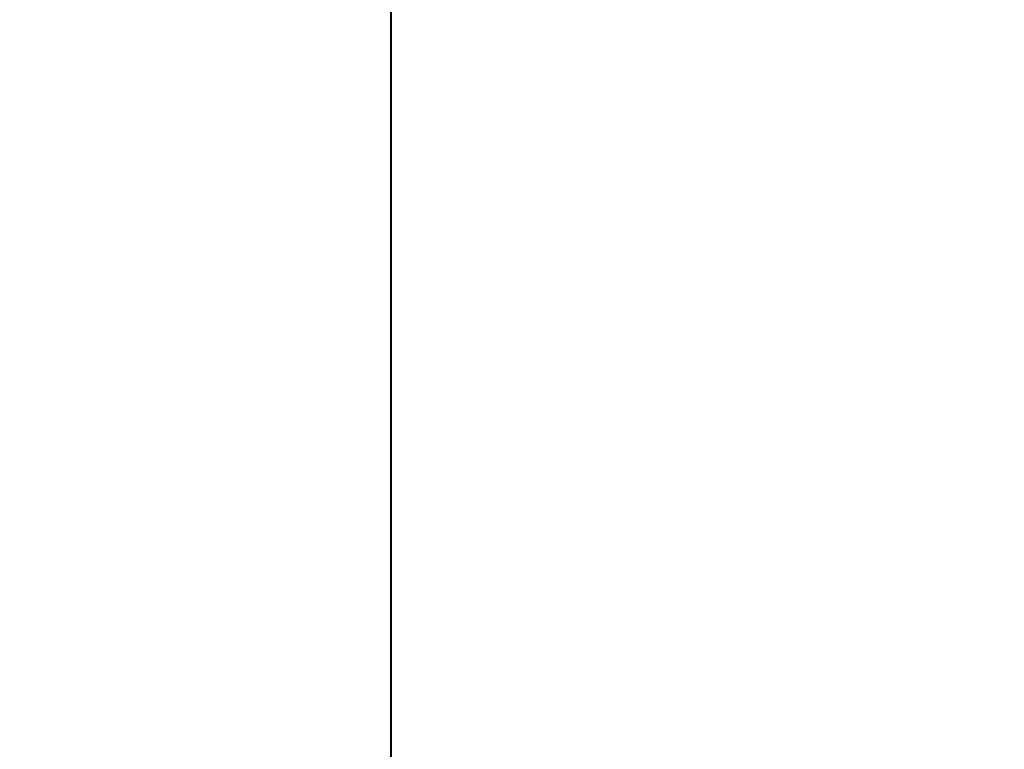
# Model space of a CAD drawing. Units: inches. Extents: x 459864 to 460310, y 324185 to 324787.
# Tile 84 of 112: x 460247.113242 to 460247.117712, y 324283.485489 to 324283.488802. Entities that reach past the tile are written whole.
import ezdxf

# ---------------------------------------------------------------- set-up
doc = ezdxf.new("R2010")
doc.units = ezdxf.units.IN
doc.layers.add('A-ANNO-DIMS', color=2, linetype='Continuous', lineweight=18)
doc.layers.add('A-WALL', color=7, linetype='Continuous', lineweight=40)
doc.styles.get("Standard").update_dxf_attribs({"font": 'arial.ttf'})
doc.dimstyles.new('ISO-25', dxfattribs={"dimtxt": 6, "dimasz": 2.5, "dimexe": 1.25, "dimexo": 0.625, "dimtad": 1, "dimdec": 1, "dimlunit": 3, "dimtxsty": 'Standard', "dimcen": 2.5, "dimadec": 0, "dimazin": 0, "dimtfac": 1, "dimtdec": 1, "dimtmove": 0, "dimatfit": 3, "dimfxl": 1, "dimarcsym": 0})

# ---------------------------------------------------------------- blocks, each defined once
blk = doc.blocks.new('*D21')
at = {"layer": 'A-ANNO-DIMS', "color": 0, "lineweight": -2, "transparency": 16777216}
for p, q in [((460247.7399266, 324715.4832328), (460309.5803685, 324715.4832328)), ((460308.3303685, 324712.9832328), (460308.3303685, 324285.9832328)), ((460247.7399266, 324283.4832328), (460309.5803685, 324283.4832328))]:
    blk.add_line(p, q, dxfattribs=at)
at = {"layer": 'A-ANNO-DIMS', "color": 0, "transparency": 16777216}
for points in [[(460307.9137019, 324712.9832328), (460308.7470352, 324712.9832328), (460308.3303685, 324715.4832328)], [(460307.9137019, 324285.9832328), (460308.7470352, 324285.9832328), (460308.3303685, 324283.4832328)]]:
    blk.add_solid(points, dxfattribs=at)
at = {"layer": 'Defpoints', "color": 0, "transparency": 16777216}
for p in [(460247.1149266, 324715.4832328), (460247.1149266, 324283.4832328), (460308.3303685, 324283.4832328)]:
    blk.add_point(p, dxfattribs=at)
at = {"layer": 'A-ANNO-DIMS', "color": 0, "transparency": 16777216, "insert": (460304.6398842, 324499.4832328), "char_height": 6, "attachment_point": 5, "rotation": 90}
blk.add_mtext("36'", dxfattribs=at)
blk = doc.blocks.new('*D62')
at = {"layer": 'A-ANNO-DIMS', "color": 0, "lineweight": -2, "transparency": 16777216}
for p, q in [((460247.739927, 324332.73872), (460278.764927, 324332.73872)), ((460277.514927, 324330.23872), (460277.514927, 324285.983233)), ((460247.739927, 324283.483233), (460278.764927, 324283.483233))]:
    blk.add_line(p, q, dxfattribs=at)
at = {"layer": 'A-ANNO-DIMS', "color": 0, "transparency": 16777216}
for points in [[(460277.0982603, 324330.23872), (460277.9315937, 324330.23872), (460277.514927, 324332.73872)], [(460277.0982603, 324285.983233), (460277.9315937, 324285.983233), (460277.514927, 324283.483233)]]:
    blk.add_solid(points, dxfattribs=at)
at = {"layer": 'Defpoints', "color": 0, "transparency": 16777216}
for p in [(460247.114927, 324332.73872), (460247.114927, 324283.483233), (460277.514927, 324283.483233)]:
    blk.add_point(p, dxfattribs=at)
at = {"layer": 'A-ANNO-DIMS', "color": 0, "transparency": 16777216, "insert": (460273.7876078, 324308.1109765), "char_height": 6, "attachment_point": 5, "rotation": 90}
blk.add_mtext('4\'-1 1/2"', dxfattribs=at)
blk = doc.blocks.new('*D67')
at = {"layer": 'A-ANNO-DIMS', "color": 0, "lineweight": -2, "transparency": 16777216}
for p, q in [((460208.114927, 324284.108233), (460208.114927, 324315.133233)), ((460247.114927, 324284.108233), (460247.114927, 324315.133233)), ((460210.614927, 324313.883233), (460244.614927, 324313.883233))]:
    blk.add_line(p, q, dxfattribs=at)
at = {"layer": 'A-ANNO-DIMS', "color": 0, "transparency": 16777216}
for points in [[(460210.614927, 324314.2998997), (460210.614927, 324313.4665663), (460208.114927, 324313.883233)], [(460244.614927, 324314.2998997), (460244.614927, 324313.4665663), (460247.114927, 324313.883233)]]:
    blk.add_solid(points, dxfattribs=at)
at = {"layer": 'Defpoints', "color": 0, "transparency": 16777216}
for p in [(460247.114927, 324313.883233), (460208.114927, 324283.483233), (460247.114927, 324283.483233)]:
    blk.add_point(p, dxfattribs=at)
at = {"layer": 'A-ANNO-DIMS', "color": 0, "transparency": 16777216, "insert": (460227.614927, 324317.5737173), "char_height": 6, "attachment_point": 5}
blk.add_mtext('3\'-3"', dxfattribs=at)

msp = doc.modelspace()

# ---------------------------------------------------------------- linework, layer by layer
at = {"layer": 'A-WALL'}
msp.add_line((460247.1149266, 324470.9832328), (460247.1149266, 324283.4832328), dxfattribs=at)

# ---------------------------------------------------------------- dimensions: what is measured, and where the dimension line sits
at = {"layer": 'A-ANNO-DIMS'}
for base, p1, p2, angle, override, picture, middle in [((460308.3303685, 324283.4832328), (460247.1149266, 324715.4832328), (460247.1149266, 324283.4832328), 90, {"dimclrd": 0, "dimclre": 0, "dimclrt": 0}, '*D21', (460304.6398842, 324499.4832328)), ((460277.514927, 324283.483233), (460247.114927, 324332.73872), (460247.114927, 324283.483233), 270, {"dimdec": 1, "dimlfac": 1, "dimrnd": 0, "dimzin": 1, "dimdsep": 46, "dimlunit": 4, "dimfrac": 2}, '*D62', (460273.7876078, 324308.1109765))]:
    dim = msp.add_linear_dim(base=base, p1=p1, p2=p2, angle=angle, dimstyle='ISO-25', override=override, dxfattribs=at)
    dim.commit()
    dim.dimension.update_dxf_attribs({"geometry": picture, "text_midpoint": middle})
dim = msp.add_linear_dim(base=(460247.114927, 324313.883233), p1=(460208.114927, 324283.483233), p2=(460247.114927, 324283.483233), dimstyle='ISO-25', override={"dimdec": 1, "dimlfac": 1, "dimrnd": 0, "dimzin": 1, "dimdsep": 46, "dimlunit": 4, "dimfrac": 2}, dxfattribs=at)
dim.commit()
dim.dimension.update_dxf_attribs({"geometry": '*D67', "text_midpoint": (460227.614927, 324317.5737173)})

doc.saveas('drawing.dxf')
